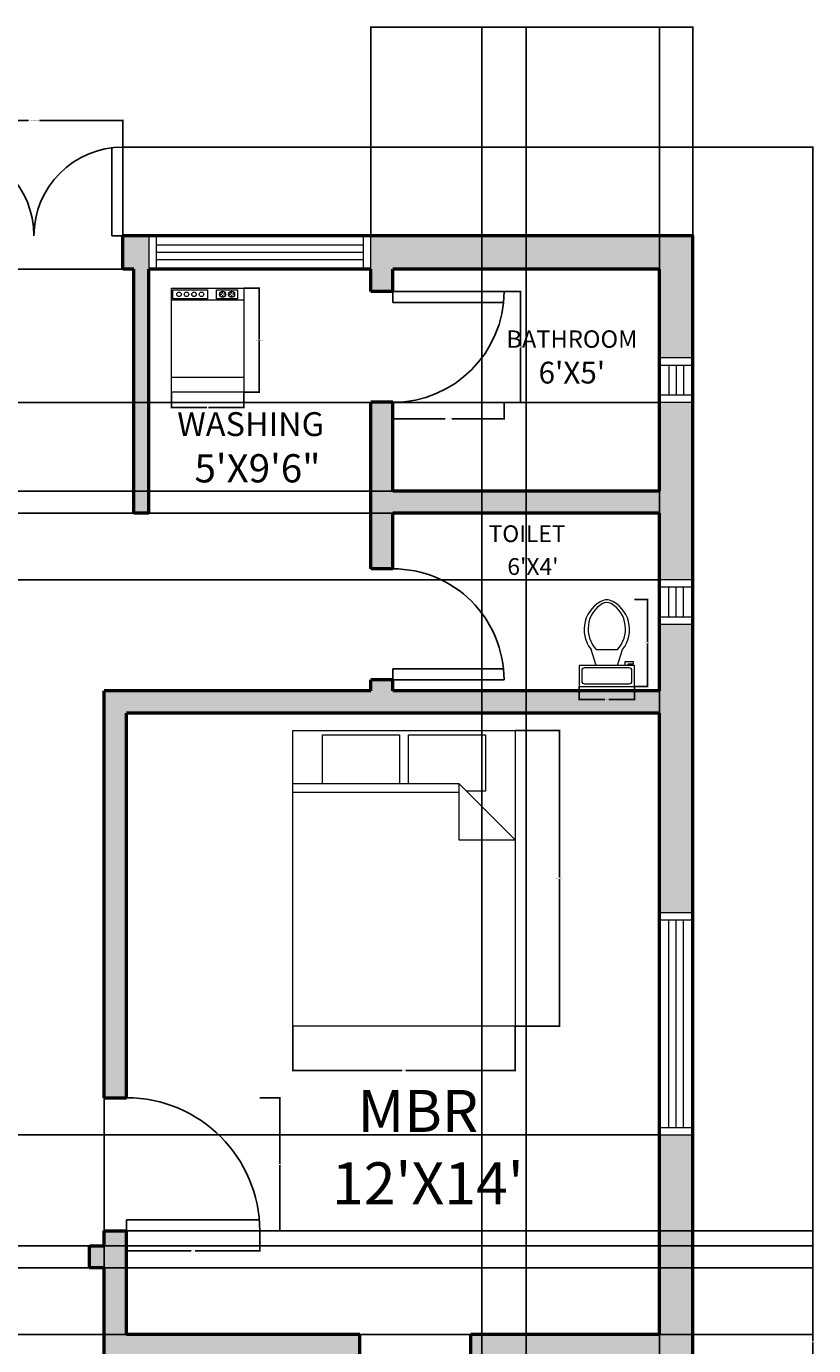
# Model space of a CAD drawing. Units: inches. Extents: x 96 to 522, y 502 to 1213.
# Tile 5 of 5: x 309 to 522, y 856 to 1213. Entities that reach past the tile are written whole.
import ezdxf

# ---------------------------------------------------------------- set-up
doc = ezdxf.new("R2010")
doc.units = ezdxf.units.IN
doc.layers.get('Defpoints').update_dxf_attribs({"color": 90})
for name, color, linetype, lineweight in [('A-ANNO-DIMS', 2, 'Continuous', 18), ('A-AREA-IDEN', 7, 'Continuous', 25), ('A-DOOR', 3, 'Continuous', 25), ('A-EQPM', 8, 'Continuous', 18), ('A-FLOR-FIXT', 9, 'Continuous', 18), ('A-FURN', 8, 'Continuous', 18), ('A-GLAZ', 4, 'Continuous', 18), ('A-WALL', 7, 'Continuous', 50)]:
    doc.layers.add(name, color=color, linetype=linetype, lineweight=lineweight)
doc.layers.add('A-WALL-PATT', color=252, linetype='Continuous', lineweight=13, true_color=0x939598)
doc.styles.get("Standard").update_dxf_attribs({"font": 'arial.ttf'})
doc.dimstyles.get("Standard").update_dxf_attribs({"dimtxt": 0.18, "dimasz": 0.18, "dimexe": 0.18, "dimexo": 0.0625, "dimgap": 0.09, "dimtad": 0, "dimtih": 1, "dimtoh": 1, "dimdec": 4, "dimzin": 0, "dimdsep": 46, "dimtxsty": 'Standard', "dimcen": 0.09, "dimadec": 0, "dimazin": 0, "dimtfac": 1, "dimtdec": 4, "dimtofl": 0, "dimtmove": 0, "dimatfit": 3, "dimfxl": 1, "dimtolj": 1, "dimtzin": 0, "dimarcsym": 0})

# ---------------------------------------------------------------- blocks, each defined once
blk = doc.blocks.new('Bed - Queen')
for p, q in [((0, -80.00003), (0, 0)), ((0, 0), (59.99999, 0)), ((59.99999, 0), (59.99999, -80.00003)), ((7.99999, -1.2), (28.79998, -1.2)), ((7.99999, -14.4), (7.99999, -1.2)), ((28.79998, -1.2), (28.79998, -14.4)), ((31.19999, -1.2), (51.99999, -1.2)), ((31.19999, -14.4), (31.19999, -1.2)), ((51.99999, -1.2), (51.99999, -16.4)), ((0, -14.4), (44.8, -14.4)), ((44.8, -16.8), (0, -16.8)), ((59.99999, -29.6), (44.8, -14.4)), ((44.8, -14.4), (44.8, -29.6)), ((51.99999, -16.4), (46.79936, -16.4)), ((44.8, -29.6), (59.99999, -29.6)), ((59.99999, -80.00003), (0, -80.00003))]:
    blk.add_line(p, q)
blk = doc.blocks.new('Toilet - top')
for p, q in [((9.5, -6), (9.5, -2)), ((-10, -8.5), (-8, -8.5)), ((-10, -9.5), (-10, -8.5)), ((-7, -9.5), (-10, -9.5)), ((-8, -8.5), (-8, -8)), ((-7, -8), (-7, -9.5)), ((-4, -8), (-6, -14)), ((4, -8), (6, -14)), ((4, -14), (-4, -14))]:
    blk.add_line(p, q)
blk.add_lwpolyline([(10.5, -8), (10.5, 0), (-10.5, 0), (-10.5, -8)], close=True)
for points in [[(-9.5, -2), (-9.5, -6)], [(8.5, -1), (-8.5, -1)], [(-8.5, -7), (8.5, -7)]]:
    blk.add_lwpolyline(points)
for centre, radius, start, end in [((-8.62, -1.88), 0.884, 81.8699, 188.1301), ((8.62, -1.88), 0.884, 351.8699, 98.1301), ((-8.62, -6.12), 0.884, 171.8699, 278.1301), ((8.62, -6.12), 0.884, 261.8699, 8.1301), ((3.52, -21.58), 12.17, 141.4691, 247.9714), ((4.2, -21.82), 11.33, 136.3677, 238.9468), ((-3.52, -21.58), 12.17, 292.0284, 38.5307), ((-4.2, -21.82), 11.33, 301.053, 43.6321), ((0, -27.88), 4, 245.7318, 294.2682), ((0, -29), 4, 254.8605, 285.1395)]:
    blk.add_arc(centre, radius, start, end)
blk = doc.blocks.new('Dishwasher')
for p, q in [((16, 32.5), (16.75, 32.5)), ((16.5, 32), (16.2942, 31.7942)), ((16.3156, 33.1843), (16.5, 33)), ((17, 32.75), (17, 33.5)), ((17, 32.25), (17, 31.5)), ((18, 32.5), (17.25, 32.5)), ((17.5, 33), (17.6938, 33.1938)), ((17.7061, 31.7939), (17.5, 32)), ((19, 32.5), (19.75, 32.5)), ((19.5, 32), (19.2942, 31.7942)), ((19.3156, 33.1843), (19.5, 33)), ((20, 32.75), (20, 33.5)), ((20, 32.25), (20, 31.5)), ((21, 32.5), (20.25, 32.5)), ((20.5, 33), (20.6938, 33.1938)), ((20.7061, 31.7939), (20.5, 32)), ((24, 30.5), (0, 30.5)), ((0, 5), (24, 5))]:
    blk.add_line(p, q)
for points in [[(0, 0), (0, 34.5), (24, 34.5), (24, 0)], [(0.5, 31), (0.5, 34), (12, 34), (12, 31)], [(15, 31), (15, 34), (22, 34), (22, 31)]]:
    blk.add_lwpolyline(points, close=True)
for centre, radius in [((2.5, 32.5), 0.75), ((5, 32.5), 0.75), ((7.5, 32.5), 0.75), ((10, 32.5), 0.75), ((17, 32.5), 1), ((20, 32.5), 1)]:
    blk.add_circle(centre, radius)
blk = doc.blocks.new('WIN-60IN')
for p, q in [((60, 9), (0, 9)), ((0, 9), (0, 0)), ((2, 9), (2, 0)), ((58, 0), (58, 9)), ((60, 0), (60, 9)), ((2, 6.5), (58, 6.5)), ((2, 4.5), (58, 4.5)), ((0, 0), (60, 0)), ((2, 2.5), (58, 2.5))]:
    blk.add_line(p, q)
blk = doc.blocks.new('WIN-12IN')
for p, q in [((0, 12), (0, 0)), ((9, 12), (0, 12)), ((9, 0), (9, 12)), ((9, 10), (0, 10)), ((2.5, 10), (2.5, 2)), ((4.5, 10), (4.5, 2)), ((6.5, 10), (6.5, 2)), ((0, 2), (9, 2)), ((0, 0), (9, 0))]:
    blk.add_line(p, q)
blk = doc.blocks.new('DOOR-SGL-36IN')
for p, q in [((36, 3), (0, 3)), ((0, 0), (0, 3)), ((36, 0), (0, 0))]:
    blk.add_line(p, q)
blk.add_arc((0, 0), 36, 0, 90)
blk = doc.blocks.new('DOOR-SGL-30IN')
for p, q in [((30, 30), (0, 30)), ((0, 30), (0, 27)), ((30, 27), (0, 27))]:
    blk.add_line(p, q)
blk.add_arc((0, 30), 30, 270, 0)
blk = doc.blocks.new('DOOR-DBL-48IN')
for p, q in [((0, 24), (0, 0)), ((3, 24), (3, 0)), ((45, 24), (45, 0)), ((48, 24), (48, 0)), ((0, 0), (3, 0)), ((48, 0), (45, 0))]:
    blk.add_line(p, q)
for centre, start, end in [((0, 0), 0, 90), ((48, 0), 90, 180)]:
    blk.add_arc(centre, 24, start, end)
blk = doc.blocks.new('*D21')
at = {"layer": 'A-ANNO-DIMS', "color": 0, "lineweight": -2, "transparency": 16777216}
for p, q in [((408.21, 1111.19), (408.21, 1106.57)), ((438.21, 1111.19), (438.21, 1106.57)), ((408.39, 1106.75), (422.28, 1106.75)), ((438.03, 1106.75), (424.15, 1106.75))]:
    blk.add_line(p, q, dxfattribs=at)
at = {"layer": 'A-ANNO-DIMS', "color": 0, "transparency": 16777216}
for points in [[(408.39, 1106.78), (408.39, 1106.72), (408.21, 1106.75)], [(438.03, 1106.78), (438.03, 1106.72), (438.21, 1106.75)]]:
    blk.add_solid(points, dxfattribs=at)
at = {"layer": 'Defpoints', "color": 0, "transparency": 16777216}
for p in [(408.21, 1111.25), (438.21, 1111.25), (438.21, 1106.75)]:
    blk.add_point(p, dxfattribs=at)
at = {"layer": 'A-ANNO-DIMS', "color": 0, "transparency": 16777216, "insert": (423.21, 1106.75), "char_height": 0.18, "attachment_point": 5}
blk.add_mtext('\\A1;DOOR 30 TYP.', dxfattribs=at)
blk = doc.blocks.new('*D22')
at = {"layer": 'A-ANNO-DIMS', "color": 0, "lineweight": -2, "transparency": 16777216}
for p, q in [((438.27, 1141.25), (442.89, 1141.25)), ((442.71, 1141.07), (442.71, 1126.43)), ((442.71, 1111.43), (442.71, 1126.07)), ((438.27, 1111.25), (442.89, 1111.25))]:
    blk.add_line(p, q, dxfattribs=at)
at = {"layer": 'A-ANNO-DIMS', "color": 0, "transparency": 16777216}
for points in [[(442.68, 1141.07), (442.74, 1141.07), (442.71, 1141.25)], [(442.68, 1111.43), (442.74, 1111.43), (442.71, 1111.25)]]:
    blk.add_solid(points, dxfattribs=at)
at = {"layer": 'Defpoints', "color": 0, "transparency": 16777216}
for p in [(438.21, 1141.25), (442.71, 1141.25), (438.21, 1111.25)]:
    blk.add_point(p, dxfattribs=at)
at = {"layer": 'A-ANNO-DIMS', "color": 0, "transparency": 16777216, "insert": (442.71, 1126.25), "char_height": 0.18, "attachment_point": 5}
blk.add_mtext('\\A1;30 TYP.', dxfattribs=at)
blk = doc.blocks.new('*D23')
at = {"layer": 'A-ANNO-DIMS', "color": 0, "lineweight": -2, "transparency": 16777216}
for p, q in [((372.27, 923.25), (377.79, 923.25)), ((377.61, 923.07), (377.61, 905.43)), ((377.61, 887.43), (377.61, 905.07)), ((372.27, 887.25), (377.79, 887.25))]:
    blk.add_line(p, q, dxfattribs=at)
at = {"layer": 'A-ANNO-DIMS', "color": 0, "transparency": 16777216}
for points in [[(377.58, 923.07), (377.64, 923.07), (377.61, 923.25)], [(377.58, 887.43), (377.64, 887.43), (377.61, 887.25)]]:
    blk.add_solid(points, dxfattribs=at)
at = {"layer": 'Defpoints', "color": 0, "transparency": 16777216}
for p in [(372.21, 923.25), (377.61, 923.25), (372.21, 887.25)]:
    blk.add_point(p, dxfattribs=at)
at = {"layer": 'A-ANNO-DIMS', "color": 0, "transparency": 16777216, "insert": (377.61, 905.25), "char_height": 0.18, "attachment_point": 5}
blk.add_mtext('\\A1;DOOR 36 TYP.', dxfattribs=at)
blk = doc.blocks.new('*D24')
at = {"layer": 'A-ANNO-DIMS', "color": 0, "lineweight": -2, "transparency": 16777216}
for p, q in [((336.21, 887.19), (336.21, 881.67)), ((372.21, 887.19), (372.21, 881.67)), ((336.39, 881.85), (353.68, 881.85)), ((372.03, 881.85), (354.74, 881.85))]:
    blk.add_line(p, q, dxfattribs=at)
at = {"layer": 'A-ANNO-DIMS', "color": 0, "transparency": 16777216}
for points in [[(336.39, 881.88), (336.39, 881.82), (336.21, 881.85)], [(372.03, 881.88), (372.03, 881.82), (372.21, 881.85)]]:
    blk.add_solid(points, dxfattribs=at)
at = {"layer": 'Defpoints', "color": 0, "transparency": 16777216}
for p in [(336.21, 887.25), (372.21, 887.25), (372.21, 881.85)]:
    blk.add_point(p, dxfattribs=at)
at = {"layer": 'A-ANNO-DIMS', "color": 0, "transparency": 16777216, "insert": (354.21, 881.85), "char_height": 0.18, "attachment_point": 5}
blk.add_mtext('\\A1;36 TYP.', dxfattribs=at)
blk = doc.blocks.new('*D25')
at = {"layer": 'A-ANNO-DIMS', "color": 0, "lineweight": -2, "transparency": 16777216}
for p, q in [((287.21, 1180.31), (287.21, 1187.63)), ((335.21, 1180.31), (335.21, 1187.63)), ((287.39, 1187.45), (309.72, 1187.45)), ((335.03, 1187.45), (312.7, 1187.45))]:
    blk.add_line(p, q, dxfattribs=at)
at = {"layer": 'A-ANNO-DIMS', "color": 0, "transparency": 16777216}
for points in [[(287.39, 1187.48), (287.39, 1187.42), (287.21, 1187.45)], [(335.03, 1187.48), (335.03, 1187.42), (335.21, 1187.45)]]:
    blk.add_solid(points, dxfattribs=at)
at = {"layer": 'Defpoints', "color": 0, "transparency": 16777216}
for p in [(335.21, 1187.45), (287.21, 1180.25), (335.21, 1180.25)]:
    blk.add_point(p, dxfattribs=at)
at = {"layer": 'A-ANNO-DIMS', "color": 0, "transparency": 16777216, "insert": (311.21, 1187.45), "char_height": 0.18, "attachment_point": 5}
blk.add_mtext('\\A1;DOUBLE DOOR 48 TYP.', dxfattribs=at)
blk = doc.blocks.new('*D27')
at = {"layer": 'A-ANNO-DIMS', "color": 0, "lineweight": -2, "transparency": 16777216}
for p, q in [((441.25, 1022.58), (453.37, 1022.58)), ((453.19, 1022.4), (453.19, 982.77)), ((453.19, 942.76), (453.19, 982.39)), ((441.25, 942.58), (453.37, 942.58))]:
    blk.add_line(p, q, dxfattribs=at)
at = {"layer": 'A-ANNO-DIMS', "color": 0, "transparency": 16777216}
for points in [[(453.16, 1022.4), (453.22, 1022.4), (453.19, 1022.58)], [(453.16, 942.76), (453.22, 942.76), (453.19, 942.58)]]:
    blk.add_solid(points, dxfattribs=at)
at = {"layer": 'Defpoints', "color": 0, "transparency": 16777216}
for p in [(441.19, 1022.58), (453.19, 1022.58), (441.19, 942.58)]:
    blk.add_point(p, dxfattribs=at)
at = {"layer": 'A-ANNO-DIMS', "color": 0, "transparency": 16777216, "insert": (453.19, 982.58), "char_height": 0.18, "attachment_point": 5}
blk.add_mtext('\\A1;QUEEN BED 80 TYP.', dxfattribs=at)
blk = doc.blocks.new('*D28')
at = {"layer": 'A-ANNO-DIMS', "color": 0, "lineweight": -2, "transparency": 16777216}
for p, q in [((381.19, 942.52), (381.19, 930.4)), ((441.19, 942.52), (441.19, 930.4)), ((381.37, 930.58), (410.66, 930.58)), ((441.01, 930.58), (411.72, 930.58))]:
    blk.add_line(p, q, dxfattribs=at)
at = {"layer": 'A-ANNO-DIMS', "color": 0, "transparency": 16777216}
for points in [[(381.37, 930.61), (381.37, 930.55), (381.19, 930.58)], [(441.01, 930.61), (441.01, 930.55), (441.19, 930.58)]]:
    blk.add_solid(points, dxfattribs=at)
at = {"layer": 'Defpoints', "color": 0, "transparency": 16777216}
for p in [(381.19, 942.58), (441.19, 942.58), (441.19, 930.58)]:
    blk.add_point(p, dxfattribs=at)
at = {"layer": 'A-ANNO-DIMS', "color": 0, "transparency": 16777216, "insert": (411.19, 930.58), "char_height": 0.18, "attachment_point": 5}
blk.add_mtext('\\A1;60 TYP.', dxfattribs=at)
blk = doc.blocks.new('*D29')
at = {"layer": 'A-ANNO-DIMS', "color": 0, "lineweight": -2, "transparency": 16777216}
for p, q in [((473.51, 1057.93), (477.15, 1057.93)), ((476.97, 1057.75), (476.97, 1046.39)), ((476.97, 1034.65), (476.97, 1046.02)), ((473.51, 1034.47), (477.15, 1034.47))]:
    blk.add_line(p, q, dxfattribs=at)
at = {"layer": 'A-ANNO-DIMS', "color": 0, "transparency": 16777216}
for points in [[(476.94, 1057.75), (477, 1057.75), (476.97, 1057.93)], [(476.94, 1034.65), (477, 1034.65), (476.97, 1034.47)]]:
    blk.add_solid(points, dxfattribs=at)
at = {"layer": 'Defpoints', "color": 0, "transparency": 16777216}
for p in [(473.45, 1057.93), (473.45, 1034.47), (476.97, 1034.47)]:
    blk.add_point(p, dxfattribs=at)
at = {"layer": 'A-ANNO-DIMS', "color": 0, "transparency": 16777216, "insert": (476.97, 1046.2), "char_height": 0.18, "attachment_point": 5}
blk.add_mtext('\\A1;WC 23 TYP.', dxfattribs=at)
blk = doc.blocks.new('*D30')
at = {"layer": 'A-ANNO-DIMS', "color": 0, "lineweight": -2, "transparency": 16777216}
for p, q in [((458.54, 1034.41), (458.54, 1030.77)), ((473.45, 1034.41), (473.45, 1030.77)), ((458.72, 1030.95), (465.48, 1030.95)), ((473.27, 1030.95), (466.51, 1030.95))]:
    blk.add_line(p, q, dxfattribs=at)
at = {"layer": 'A-ANNO-DIMS', "color": 0, "transparency": 16777216}
for points in [[(458.72, 1030.98), (458.72, 1030.92), (458.54, 1030.95)], [(473.27, 1030.98), (473.27, 1030.92), (473.45, 1030.95)]]:
    blk.add_solid(points, dxfattribs=at)
at = {"layer": 'Defpoints', "color": 0, "transparency": 16777216}
for p in [(458.54, 1034.47), (473.45, 1034.47), (458.54, 1030.95)]:
    blk.add_point(p, dxfattribs=at)
at = {"layer": 'A-ANNO-DIMS', "color": 0, "transparency": 16777216, "insert": (466, 1030.95), "char_height": 0.18, "attachment_point": 5}
blk.add_mtext('\\A1;15 TYP.', dxfattribs=at)
blk = doc.blocks.new('*D43')
at = {"layer": 'A-ANNO-DIMS', "color": 0, "lineweight": -2, "transparency": 16777216}
for p, q in [((367.93, 1142.08), (372.26, 1142.08)), ((372.08, 1141.9), (372.08, 1128.23)), ((372.08, 1114.2), (372.08, 1127.87)), ((367.93, 1114.02), (372.26, 1114.02))]:
    blk.add_line(p, q, dxfattribs=at)
at = {"layer": 'A-ANNO-DIMS', "color": 0, "transparency": 16777216}
for points in [[(372.05, 1141.9), (372.11, 1141.9), (372.08, 1142.08)], [(372.05, 1114.2), (372.11, 1114.2), (372.08, 1114.02)]]:
    blk.add_solid(points, dxfattribs=at)
at = {"layer": 'Defpoints', "color": 0, "transparency": 16777216}
for p in [(367.87, 1142.08), (372.08, 1142.08), (367.87, 1114.02)]:
    blk.add_point(p, dxfattribs=at)
at = {"layer": 'A-ANNO-DIMS', "color": 0, "transparency": 16777216, "insert": (372.08, 1128.05), "char_height": 0.18, "attachment_point": 5}
blk.add_mtext('\\A1;DISHWASHER 28', dxfattribs=at)
blk = doc.blocks.new('*D44')
at = {"layer": 'A-ANNO-DIMS', "color": 0, "lineweight": -2, "transparency": 16777216}
for p, q in [((348.35, 1113.96), (348.35, 1109.63)), ((367.87, 1113.96), (367.87, 1109.63)), ((348.53, 1109.81), (357.89, 1109.81)), ((367.69, 1109.81), (358.33, 1109.81))]:
    blk.add_line(p, q, dxfattribs=at)
at = {"layer": 'A-ANNO-DIMS', "color": 0, "transparency": 16777216}
for points in [[(348.53, 1109.84), (348.53, 1109.78), (348.35, 1109.81)], [(367.69, 1109.84), (367.69, 1109.78), (367.87, 1109.81)]]:
    blk.add_solid(points, dxfattribs=at)
at = {"layer": 'Defpoints', "color": 0, "transparency": 16777216}
for p in [(348.35, 1114.02), (367.87, 1114.02), (367.87, 1109.81)]:
    blk.add_point(p, dxfattribs=at)
at = {"layer": 'A-ANNO-DIMS', "color": 0, "transparency": 16777216, "insert": (358.11, 1109.81), "char_height": 0.18, "attachment_point": 5}
blk.add_mtext('\\A1;20', dxfattribs=at)
blk = doc.blocks.new('*D48')
at = {"layer": 'A-ANNO-DIMS', "color": 0, "lineweight": -2, "transparency": 16777216}
for p, q in [((335.27, 1180.25), (521.84, 1180.25)), ((521.66, 1180.07), (521.66, 857.43)), ((521.66, 534.43), (521.66, 857.07)), ((489.27, 534.25), (521.84, 534.25))]:
    blk.add_line(p, q, dxfattribs=at)
at = {"layer": 'A-ANNO-DIMS', "color": 0, "transparency": 16777216}
for points in [[(521.63, 1180.07), (521.69, 1180.07), (521.66, 1180.25)], [(521.63, 534.43), (521.69, 534.43), (521.66, 534.25)]]:
    blk.add_solid(points, dxfattribs=at)
at = {"layer": 'Defpoints', "color": 0, "transparency": 16777216}
for p in [(335.21, 1180.25), (521.66, 1180.25), (489.21, 534.25)]:
    blk.add_point(p, dxfattribs=at)
at = {"layer": 'A-ANNO-DIMS', "color": 0, "transparency": 16777216, "insert": (521.66, 857.25), "char_height": 0.18, "attachment_point": 5}
blk.add_mtext('\\A1;646', dxfattribs=at)
blk = doc.blocks.new('*D52')
at = {"layer": 'A-ANNO-DIMS', "color": 0, "lineweight": -2, "transparency": 16777216}
for p, q in [((402.21, 1156.31), (402.21, 1212.88)), ((402.39, 1212.7), (445.49, 1212.7)), ((489.03, 1212.7), (445.93, 1212.7)), ((489.21, 1156.31), (489.21, 1212.88))]:
    blk.add_line(p, q, dxfattribs=at)
at = {"layer": 'A-ANNO-DIMS', "color": 0, "transparency": 16777216}
for points in [[(402.39, 1212.73), (402.39, 1212.67), (402.21, 1212.7)], [(489.03, 1212.73), (489.03, 1212.67), (489.21, 1212.7)]]:
    blk.add_solid(points, dxfattribs=at)
at = {"layer": 'Defpoints', "color": 0, "transparency": 16777216}
for p in [(489.21, 1212.7), (402.21, 1156.25), (489.21, 1156.25)]:
    blk.add_point(p, dxfattribs=at)
at = {"layer": 'A-ANNO-DIMS', "color": 0, "transparency": 16777216, "insert": (445.71, 1212.7), "char_height": 0.18, "attachment_point": 5}
blk.add_mtext('\\A1;87', dxfattribs=at)
blk = doc.blocks.new('*D55')
at = {"layer": 'A-ANNO-DIMS', "color": 0, "lineweight": -2, "transparency": 16777216}
for p, q in [((432.21, 661.31), (432.21, 1212.88)), ((432.39, 1212.7), (455.99, 1212.7)), ((480.03, 1212.7), (456.43, 1212.7)), ((480.21, 661.31), (480.21, 1212.88))]:
    blk.add_line(p, q, dxfattribs=at)
at = {"layer": 'A-ANNO-DIMS', "color": 0, "transparency": 16777216}
for points in [[(432.39, 1212.73), (432.39, 1212.67), (432.21, 1212.7)], [(480.03, 1212.73), (480.03, 1212.67), (480.21, 1212.7)]]:
    blk.add_solid(points, dxfattribs=at)
at = {"layer": 'Defpoints', "color": 0, "transparency": 16777216}
for p in [(480.21, 1212.7), (432.21, 661.25), (480.21, 661.25)]:
    blk.add_point(p, dxfattribs=at)
at = {"layer": 'A-ANNO-DIMS', "color": 0, "transparency": 16777216, "insert": (456.21, 1212.7), "char_height": 0.18, "attachment_point": 5}
blk.add_mtext('\\A1;48', dxfattribs=at)
blk = doc.blocks.new('*D62')
at = {"layer": 'A-ANNO-DIMS', "color": 0, "lineweight": -2, "transparency": 16777216}
for p, q in [((480.15, 913.25), (96.58, 913.25)), ((96.76, 913.07), (96.76, 886.43)), ((96.76, 859.43), (96.76, 886.07)), ((480.15, 859.25), (96.58, 859.25))]:
    blk.add_line(p, q, dxfattribs=at)
at = {"layer": 'A-ANNO-DIMS', "color": 0, "transparency": 16777216}
for points in [[(96.73, 913.07), (96.79, 913.07), (96.76, 913.25)], [(96.73, 859.43), (96.79, 859.43), (96.76, 859.25)]]:
    blk.add_solid(points, dxfattribs=at)
at = {"layer": 'Defpoints', "color": 0, "transparency": 16777216}
for p in [(96.76, 913.25), (480.21, 913.25), (480.21, 859.25)]:
    blk.add_point(p, dxfattribs=at)
at = {"layer": 'A-ANNO-DIMS', "color": 0, "transparency": 16777216, "insert": (96.76, 886.25), "char_height": 0.18, "attachment_point": 5}
blk.add_mtext('\\A1;54', dxfattribs=at)
blk = doc.blocks.new('*D63')
at = {"layer": 'A-ANNO-DIMS', "color": 0, "lineweight": -2, "transparency": 16777216}
for p, q in [((480.15, 1081.25), (96.58, 1081.25)), ((96.76, 1081.07), (96.76, 1072.43)), ((96.76, 1063.43), (96.76, 1072.07)), ((480.15, 1063.25), (96.58, 1063.25))]:
    blk.add_line(p, q, dxfattribs=at)
at = {"layer": 'A-ANNO-DIMS', "color": 0, "transparency": 16777216}
for points in [[(96.73, 1081.07), (96.79, 1081.07), (96.76, 1081.25)], [(96.73, 1063.43), (96.79, 1063.43), (96.76, 1063.25)]]:
    blk.add_solid(points, dxfattribs=at)
at = {"layer": 'Defpoints', "color": 0, "transparency": 16777216}
for p in [(96.76, 1081.25), (480.21, 1081.25), (480.21, 1063.25)]:
    blk.add_point(p, dxfattribs=at)
at = {"layer": 'A-ANNO-DIMS', "color": 0, "transparency": 16777216, "insert": (96.76, 1072.25), "char_height": 0.18, "attachment_point": 5}
blk.add_mtext('\\A1;18', dxfattribs=at)
blk = doc.blocks.new('*D64')
at = {"layer": 'A-ANNO-DIMS', "color": 0, "lineweight": -2, "transparency": 16777216}
for p, q in [((480.15, 1111.25), (96.58, 1111.25)), ((96.76, 1111.07), (96.76, 1099.43)), ((96.76, 1087.43), (96.76, 1099.07)), ((480.15, 1087.25), (96.58, 1087.25))]:
    blk.add_line(p, q, dxfattribs=at)
at = {"layer": 'A-ANNO-DIMS', "color": 0, "transparency": 16777216}
for points in [[(96.73, 1111.07), (96.79, 1111.07), (96.76, 1111.25)], [(96.73, 1087.43), (96.79, 1087.43), (96.76, 1087.25)]]:
    blk.add_solid(points, dxfattribs=at)
at = {"layer": 'Defpoints', "color": 0, "transparency": 16777216}
for p in [(96.76, 1111.25), (480.21, 1111.25), (480.21, 1087.25)]:
    blk.add_point(p, dxfattribs=at)
at = {"layer": 'A-ANNO-DIMS', "color": 0, "transparency": 16777216, "insert": (96.76, 1099.25), "char_height": 0.18, "attachment_point": 5}
blk.add_mtext('\\A1;24', dxfattribs=at)
blk = doc.blocks.new('*D65')
at = {"layer": 'A-ANNO-DIMS', "color": 0, "lineweight": -2, "transparency": 16777216}
for p, q in [((444.21, 543.31), (444.21, 1212.88)), ((444.39, 1212.7), (461.99, 1212.7)), ((480.03, 1212.7), (462.43, 1212.7)), ((480.21, 543.31), (480.21, 1212.88))]:
    blk.add_line(p, q, dxfattribs=at)
at = {"layer": 'A-ANNO-DIMS', "color": 0, "transparency": 16777216}
for points in [[(444.39, 1212.73), (444.39, 1212.67), (444.21, 1212.7)], [(480.03, 1212.73), (480.03, 1212.67), (480.21, 1212.7)]]:
    blk.add_solid(points, dxfattribs=at)
at = {"layer": 'Defpoints', "color": 0, "transparency": 16777216}
for p in [(480.21, 1212.7), (444.21, 543.25), (480.21, 543.25)]:
    blk.add_point(p, dxfattribs=at)
at = {"layer": 'A-ANNO-DIMS', "color": 0, "transparency": 16777216, "insert": (462.21, 1212.7), "char_height": 0.18, "attachment_point": 5}
blk.add_mtext('\\A1;36', dxfattribs=at)
blk = doc.blocks.new('*D66')
at = {"layer": 'A-ANNO-DIMS', "color": 0, "lineweight": -2, "transparency": 16777216}
for p, q in [((330.21, 1033.19), (330.21, 501.62)), ((276.21, 997.19), (276.21, 501.62)), ((276.39, 501.8), (302.99, 501.8)), ((330.03, 501.8), (303.43, 501.8))]:
    blk.add_line(p, q, dxfattribs=at)
at = {"layer": 'A-ANNO-DIMS', "color": 0, "transparency": 16777216}
for points in [[(276.39, 501.83), (276.39, 501.77), (276.21, 501.8)], [(330.03, 501.83), (330.03, 501.77), (330.21, 501.8)]]:
    blk.add_solid(points, dxfattribs=at)
at = {"layer": 'Defpoints', "color": 0, "transparency": 16777216}
for p in [(330.21, 1033.25), (276.21, 997.25), (330.21, 501.8)]:
    blk.add_point(p, dxfattribs=at)
at = {"layer": 'A-ANNO-DIMS', "color": 0, "transparency": 16777216, "insert": (303.21, 501.8), "char_height": 0.18, "attachment_point": 5}
blk.add_mtext('\\A1;54', dxfattribs=at)
blk = doc.blocks.new('*D67')
at = {"layer": 'A-ANNO-DIMS', "color": 0, "lineweight": -2, "transparency": 16777216}
for p, q in [((276.27, 883.25), (521.84, 883.25)), ((521.66, 883.07), (521.66, 880.43)), ((521.66, 877.43), (521.66, 880.07)), ((276.27, 877.25), (521.84, 877.25))]:
    blk.add_line(p, q, dxfattribs=at)
at = {"layer": 'A-ANNO-DIMS', "color": 0, "transparency": 16777216}
for points in [[(521.63, 883.07), (521.69, 883.07), (521.66, 883.25)], [(521.63, 877.43), (521.69, 877.43), (521.66, 877.25)]]:
    blk.add_solid(points, dxfattribs=at)
at = {"layer": 'Defpoints', "color": 0, "transparency": 16777216}
for p in [(276.21, 883.25), (521.66, 883.25), (276.21, 877.25)]:
    blk.add_point(p, dxfattribs=at)
at = {"layer": 'A-ANNO-DIMS', "color": 0, "transparency": 16777216, "insert": (521.66, 880.25), "char_height": 0.18, "attachment_point": 5}
blk.add_mtext('\\A1;6', dxfattribs=at)
blk = doc.blocks.new('*D68')
at = {"layer": 'A-ANNO-DIMS', "color": 0, "lineweight": -2, "transparency": 16777216}
for p, q in [((336.27, 887.25), (521.84, 887.25)), ((521.66, 887.07), (521.66, 873.43)), ((521.66, 859.43), (521.66, 873.07)), ((336.27, 859.25), (521.84, 859.25))]:
    blk.add_line(p, q, dxfattribs=at)
at = {"layer": 'A-ANNO-DIMS', "color": 0, "transparency": 16777216}
for points in [[(521.63, 887.07), (521.69, 887.07), (521.66, 887.25)], [(521.63, 859.43), (521.69, 859.43), (521.66, 859.25)]]:
    blk.add_solid(points, dxfattribs=at)
at = {"layer": 'Defpoints', "color": 0, "transparency": 16777216}
for p in [(336.21, 887.25), (521.66, 887.25), (336.21, 859.25)]:
    blk.add_point(p, dxfattribs=at)
at = {"layer": 'A-ANNO-DIMS', "color": 0, "transparency": 16777216, "insert": (521.66, 873.25), "char_height": 0.18, "attachment_point": 5}
blk.add_mtext('\\A1;28', dxfattribs=at)
blk = doc.blocks.new('*D71')
at = {"layer": 'A-ANNO-DIMS', "color": 0, "lineweight": -2, "transparency": 16777216}
for p, q in [((338.15, 1147.25), (96.58, 1147.25)), ((96.76, 1147.07), (96.76, 1114.43)), ((96.76, 1081.43), (96.76, 1114.07)), ((338.15, 1081.25), (96.58, 1081.25))]:
    blk.add_line(p, q, dxfattribs=at)
at = {"layer": 'A-ANNO-DIMS', "color": 0, "transparency": 16777216}
for points in [[(96.73, 1147.07), (96.79, 1147.07), (96.76, 1147.25)], [(96.73, 1081.43), (96.79, 1081.43), (96.76, 1081.25)]]:
    blk.add_solid(points, dxfattribs=at)
at = {"layer": 'Defpoints', "color": 0, "transparency": 16777216}
for p in [(96.76, 1147.25), (338.21, 1147.25), (338.21, 1081.25)]:
    blk.add_point(p, dxfattribs=at)
at = {"layer": 'A-ANNO-DIMS', "color": 0, "transparency": 16777216, "insert": (96.76, 1114.25), "char_height": 0.18, "attachment_point": 5}
blk.add_mtext('\\A1;66', dxfattribs=at)

msp = doc.modelspace()

# ---------------------------------------------------------------- hatches: boundary and pattern name
at = {"layer": 'A-WALL-PATT'}
h = msp.add_hatch(color=256, dxfattribs=at)
h.dxf.hatch_style = 1
h.paths.add_polyline_path([(174.2111, 1156.2511), (129.2111, 1156.2511), (129.2111, 1105.2511), (138.2111, 1105.2511), (138.2111, 1147.2511), (174.2111, 1147.2511)])
h.paths.add_polyline_path([(287.2111, 1156.2511), (234.2111, 1156.2511), (234.2111, 1147.2511), (270.2111, 1147.2511), (270.2111, 1003.2511), (267.2111, 1003.2511), (267.2111, 997.2511), (276.2111, 997.2511), (276.2111, 1147.2511), (287.2111, 1147.2511)])
h.paths.add_polyline_path([(342.2111, 1156.2511), (335.2111, 1156.2511), (335.2111, 1147.2511), (338.2111, 1147.2511), (338.2111, 1081.2511), (342.2111, 1081.2511), (342.2111, 1147.2511)])
h.paths.add_polyline_path([(489.2111, 1156.2511), (402.2111, 1156.2511), (402.2111, 1147.2511), (402.2111, 1141.2511), (408.2111, 1141.2511), (408.2111, 1147.2511), (480.2111, 1147.2511), (480.2111, 1123.2511), (489.2111, 1123.2511)])
h.paths.add_polyline_path([(489.2111, 1111.2511), (480.2111, 1111.2511), (480.2111, 1087.2511), (408.2111, 1087.2511), (408.2111, 1111.2511), (402.2111, 1111.2511), (402.2111, 1066.2511), (408.2111, 1066.2511), (408.2111, 1081.2511), (480.2111, 1081.2511), (480.2111, 1063.2511), (489.2111, 1063.2511)])
h.paths.add_polyline_path([(489.2111, 1051.2511), (480.2111, 1051.2511), (480.2111, 1033.2511), (408.2111, 1033.2511), (408.2111, 1036.2511), (402.2111, 1036.2511), (402.2111, 1033.2511), (338.2111, 1033.2511), (330.2111, 1033.2511), (330.2111, 923.2511), (336.2111, 923.2511), (336.2111, 1027.2511), (338.2111, 1027.2511), (402.2111, 1027.2511), (480.2111, 1027.2511), (480.2111, 973.2511), (489.2111, 973.2511)])
h.paths.add_polyline_path([(489.2111, 913.2511), (480.2111, 913.2511), (480.2111, 859.2511), (429.2111, 859.2511), (429.2111, 853.2511), (480.2111, 853.2511), (480.2111, 829.2511), (489.2111, 829.2511)])
h.paths.add_polyline_path([(489.2111, 817.2511), (480.2111, 817.2511), (480.2111, 793.2511), (402.2111, 793.2511), (396.2111, 793.2511), (396.2111, 853.2511), (399.2111, 853.2511), (399.2111, 859.2511), (338.2111, 859.2511), (336.2111, 859.2511), (336.2111, 877.2511), (336.2111, 883.2511), (336.2111, 887.2511), (330.2111, 887.2511), (330.2111, 883.2511), (326.2111, 883.2511), (326.2111, 877.2511), (330.2111, 877.2511), (330.2111, 853.2511), (338.2111, 853.2511), (390.2111, 853.2511), (390.2111, 793.2511), (387.2111, 793.2511), (387.2111, 787.2511), (402.2111, 787.2511), (480.2111, 787.2511), (480.2111, 754.2511), (489.2111, 754.2511)])
h.paths.add_polyline_path([(489.2111, 694.2511), (480.2111, 694.2511), (480.2111, 661.2511), (432.2111, 661.2511), (432.2111, 652.2511), (480.2111, 652.2511), (480.2111, 543.2511), (333.2111, 543.2511), (333.2111, 534.2511), (489.2111, 534.2511), (489.2111, 652.2511)])
h.paths.add_polyline_path([(372.2111, 661.2511), (336.2111, 661.2511), (336.2111, 787.2511), (338.2111, 787.2511), (351.2111, 787.2511), (351.2111, 793.2511), (338.2111, 793.2511), (330.2111, 793.2511), (330.2111, 661.2511), (324.2111, 661.2511), (324.2111, 652.2511), (372.2111, 652.2511)])
h.paths.add_polyline_path([(138.2111, 680.6946), (129.2111, 680.6946), (129.2111, 652.2511), (177.2111, 652.2511), (177.2111, 661.2511), (138.2111, 661.2511)])
h.paths.add_polyline_path([(276.2111, 661.2511), (237.2111, 661.2511), (237.2111, 652.2511), (276.2111, 652.2511)])
h.paths.add_polyline_path([(138.2111, 803.1393), (129.2111, 803.1393), (129.2111, 740.6946), (138.2111, 740.6946)])
h.paths.add_polyline_path([(138.2111, 907.2511), (129.2111, 907.2511), (129.2111, 863.1393), (138.2111, 863.1393), (138.2111, 877.2511), (276.2111, 877.2511), (276.2111, 883.2511), (204.2111, 883.2511), (204.2111, 886.2511), (198.2111, 886.2511), (198.2111, 883.2511), (138.2111, 883.2511)])
h.paths.add_polyline_path([(138.2111, 943.2511), (198.2111, 943.2511), (198.2111, 916.2511), (204.2111, 916.2511), (204.2111, 949.2511), (138.2111, 949.2511), (138.2111, 997.2511), (231.2111, 997.2511), (231.2111, 1003.2511), (138.2111, 1003.2511), (138.2111, 1045.2511), (129.2111, 1045.2511), (129.2111, 919.2511), (138.2111, 919.2511)])

# ---------------------------------------------------------------- linework, layer by layer
at = {"layer": 'A-WALL'}
for p, q in [((335.2111, 1147.2511), (335.2111, 1156.2511)), ((338.2111, 1147.2511), (335.2111, 1147.2511)), ((338.2111, 1081.2511), (338.2111, 1147.2511)), ((342.2111, 1081.2511), (342.2111, 1147.2511)), ((402.2111, 1147.2511), (342.2111, 1147.2511)), ((402.2111, 1141.2511), (402.2111, 1147.2511)), ((480.2111, 1147.2511), (408.2111, 1147.2511)), ((408.2111, 1141.2511), (408.2111, 1147.2511)), ((480.2111, 1087.2511), (480.2111, 1147.2511)), ((408.2111, 1141.2511), (402.2111, 1141.2511)), ((408.2111, 1111.2511), (402.2111, 1111.2511)), ((402.2111, 1066.2511), (402.2111, 1111.2511)), ((408.2111, 1087.2511), (408.2111, 1111.2511)), ((480.2111, 1087.2511), (408.2111, 1087.2511)), ((342.2111, 1081.2511), (338.2111, 1081.2511)), ((480.2111, 1081.2511), (408.2111, 1081.2511)), ((408.2111, 1066.2511), (408.2111, 1081.2511)), ((480.2111, 1033.2511), (480.2111, 1081.2511)), ((408.2111, 1066.2511), (402.2111, 1066.2511)), ((402.2111, 1033.2511), (402.2111, 1036.2511)), ((408.2111, 1036.2511), (402.2111, 1036.2511)), ((408.2111, 1033.2511), (408.2111, 1036.2511)), ((338.2111, 1033.2511), (330.2111, 1033.2511)), ((330.2111, 923.2511), (330.2111, 1033.2511)), ((402.2111, 1033.2511), (338.2111, 1033.2511)), ((480.2111, 1033.2511), (408.2111, 1033.2511)), ((338.2111, 1027.2511), (336.2111, 1027.2511)), ((336.2111, 923.2511), (336.2111, 1027.2511)), ((402.2111, 1027.2511), (338.2111, 1027.2511)), ((480.2111, 1027.2511), (402.2111, 1027.2511)), ((480.2111, 859.2511), (480.2111, 1027.2511)), ((330.2111, 923.2511), (336.2111, 923.2511)), ((330.2111, 883.2511), (330.2111, 887.2511)), ((330.2111, 887.2511), (336.2111, 887.2511)), ((336.2111, 883.2511), (336.2111, 887.2511)), ((326.2111, 883.2511), (330.2111, 883.2511)), ((326.2111, 877.2511), (326.2111, 883.2511)), ((336.2111, 877.2511), (336.2111, 883.2511)), ((330.2111, 877.2511), (326.2111, 877.2511)), ((330.2111, 853.2511), (330.2111, 877.2511)), ((336.2111, 859.2511), (336.2111, 877.2511)), ((338.2111, 859.2511), (336.2111, 859.2511)), ((399.2111, 859.2511), (338.2111, 859.2511)), ((399.2111, 853.2511), (399.2111, 859.2511)), ((480.2111, 859.2511), (429.2111, 859.2511)), ((429.2111, 853.2511), (429.2111, 859.2511))]:
    msp.add_line(p, q, dxfattribs=at)
msp.add_lwpolyline([(489.2111, 652.2511), (489.2111, 1156.2511), (335.2111, 1156.2511)], dxfattribs=at)

# ---------------------------------------------------------------- block references
at = {"layer": 'A-DOOR'}
for name, p in [('DOOR-DBL-48IN', (287.2111, 1156.2511)), ('DOOR-SGL-30IN', (408.2111, 1111.2511)), ('DOOR-SGL-36IN', (336.2111, 887.2511))]:
    msp.add_blockref(name, p, dxfattribs=at)
at = {"layer": 'A-DOOR', "extrusion": (0, 0, -1), "zscale": -1, "rotation": 180}
msp.add_blockref('DOOR-SGL-30IN', (-408.2111, 1066.2511), dxfattribs=at)
at = {"layer": 'A-EQPM', "xscale": 0.8133739301209052, "yscale": 0.8133739301209052, "zscale": 0.8133739301209052}
msp.add_blockref('Dishwasher', (348.3483, 1114.0182), dxfattribs=at)
at = {"layer": 'A-FLOR-FIXT', "xscale": 0.7100067742046297, "yscale": 0.7100067742046297, "zscale": 0.7100067742046297, "rotation": 180}
msp.add_blockref('Toilet - top', (465.9953, 1034.4712), dxfattribs=at)
at = {"layer": 'A-FURN'}
msp.add_blockref('Bed - Queen', (381.1925, 1022.5798), dxfattribs=at)
at = {"layer": 'A-GLAZ'}
for name, p, rotation in [('WIN-60IN', (402.2111, 1156.2511), 180), ('WIN-12IN', (489.2111, 1063.2511), 180), ('WIN-60IN', (489.2111, 913.2511), 89.99999999999969)]:
    msp.add_blockref(name, p, dxfattribs=dict(at, rotation=rotation))
msp.add_blockref('WIN-12IN', (480.2111, 1111.2511), dxfattribs=at)

# ---------------------------------------------------------------- texts
at = {"layer": 'A-AREA-IDEN', "attachment_point": 1}
for s, width, gutter_width, insert, char_height in [('BATHROOM', 25.771626, 23.4992, (438.836, 1130.6985), 4.69985), ("6'X5'", 32.262638, 29.4179, (447.5484, 1122.22), 5.88358), ('WASHING', 35.31129, 32.1978, (349.9167, 1108.5818), 6.43955), ('5\'X9\'6"', 41.857968, 38.1672, (354.5849, 1097.2374), 7.63344), ('TOILET', 24.813541, 22.6256, (434.0476, 1078.0005), 4.52513), ("6'X4'", 24.813541, 22.6256, (439.1136, 1069.1261), 4.52513), ('MBR', 62.228554, 56.7416, (398.6824, 925.364), 11.34833), ("12'X14'", 62.228554, 56.7416, (391.707, 905.8), 11.34833)]:
    msp.add_mtext_dynamic_manual_height_columns(s, width=width, gutter_width=gutter_width, heights=[0], dxfattribs=dict(at, insert=insert, char_height=char_height))

# ---------------------------------------------------------------- dimensions: what is measured, and where the dimension line sits
at = {"layer": 'A-ANNO-DIMS'}
for base, p1, p2, picture, middle in [((489.2111, 1212.7011), (402.2111, 1156.2511), (489.2111, 1156.2511), '*D52', (445.7111, 1212.7011)), ((480.2111, 1212.7011), (432.2111, 661.2511), (480.2111, 661.2511), '*D55', (456.2111, 1212.7011)), ((480.2111, 1212.7011), (444.2111, 543.2511), (480.2111, 543.2511), '*D65', (462.2111, 1212.7011)), ((367.8693, 1109.809), (348.3483, 1114.0182), (367.8693, 1114.0182), '*D44', (358.1088, 1109.809)), ((330.2111, 501.8011), (276.2111, 997.2511), (330.2111, 1033.2511), '*D66', (303.2111, 501.8011))]:
    dim = msp.add_linear_dim(base=base, p1=p1, p2=p2, dimstyle='Standard', override={"dimdec": 0, "dimlfac": 1, "dimrnd": 0, "dimzin": 0, "dimdsep": 46, "dimlunit": 2}, dxfattribs=at)
    dim.commit()
    dim.dimension.update_dxf_attribs({"geometry": picture, "text_midpoint": middle})
for base, p1, p2, text, picture, middle in [((335.2111, 1187.4511), (287.2111, 1180.2511), (335.2111, 1180.2511), 'DOUBLE DOOR <> TYP.', '*D25', (311.2111, 1187.4511)), ((438.2111, 1106.7511), (408.2111, 1111.2511), (438.2111, 1111.2511), 'DOOR <> TYP.', '*D21', (423.2111, 1106.7511)), ((441.1925, 930.5798), (381.1925, 942.5798), (441.1925, 942.5798), '<> TYP.', '*D28', (411.1925, 930.5798)), ((372.2111, 881.8511), (336.2111, 887.2511), (372.2111, 887.2511), '<> TYP.', '*D24', (354.2111, 881.8511))]:
    dim = msp.add_linear_dim(base=base, p1=p1, p2=p2, text=text, dimstyle='Standard', override={"dimdec": 0, "dimlfac": 1, "dimrnd": 0, "dimzin": 0, "dimdsep": 46, "dimlunit": 2}, dxfattribs=at)
    dim.commit()
    dim.dimension.update_dxf_attribs({"geometry": picture, "text_midpoint": middle})
for base, p1, p2, picture, middle in [((521.6611, 1180.2511), (489.2111, 534.2511), (335.2111, 1180.2511), '*D48', (521.6611, 857.2511)), ((96.7611, 1147.2511), (338.2111, 1081.2511), (338.2111, 1147.2511), '*D71', (96.7611, 1114.2511)), ((96.7611, 1111.2511), (480.2111, 1087.2511), (480.2111, 1111.2511), '*D64', (96.7611, 1099.2511)), ((96.7611, 1081.2511), (480.2111, 1063.2511), (480.2111, 1081.2511), '*D63', (96.7611, 1072.2511)), ((96.7611, 913.2511), (480.2111, 859.2511), (480.2111, 913.2511), '*D62', (96.7611, 886.2511)), ((521.6611, 887.2511), (336.2111, 859.2511), (336.2111, 887.2511), '*D68', (521.6611, 873.2511)), ((521.6611, 883.2511), (276.2111, 877.2511), (276.2111, 883.2511), '*D67', (521.6611, 880.2511))]:
    dim = msp.add_linear_dim(base=base, p1=p1, p2=p2, angle=90, dimstyle='Standard', override={"dimdec": 0, "dimlfac": 1, "dimrnd": 0, "dimzin": 0, "dimdsep": 46, "dimlunit": 2}, dxfattribs=at)
    dim.commit()
    dim.dimension.update_dxf_attribs({"geometry": picture, "text_midpoint": middle})
for base, p1, p2, angle, text, picture, middle in [((372.0785, 1142.0796), (367.8693, 1114.0182), (367.8693, 1142.0796), 90, 'DISHWASHER <>', '*D43', (372.0785, 1128.0489)), ((442.7111, 1141.2511), (438.2111, 1111.2511), (438.2111, 1141.2511), 90, '<> TYP.', '*D22', (442.7111, 1126.2511)), ((476.9698, 1034.4712), (473.4503, 1057.9343), (473.4503, 1034.4712), 270, 'WC <> TYP.', '*D29', (476.9698, 1046.2028)), ((458.5402, 1030.9518), (473.4503, 1034.4712), (458.5402, 1034.4712), 180, '<> TYP.', '*D30', (465.9953, 1030.9518)), ((453.1925, 1022.5798), (441.1925, 942.5798), (441.1925, 1022.5798), 90, 'QUEEN BED <> TYP.', '*D27', (453.1925, 982.5798)), ((377.6111, 923.2511), (372.2111, 887.2511), (372.2111, 923.2511), 90, 'DOOR <> TYP.', '*D23', (377.6111, 905.2511))]:
    dim = msp.add_linear_dim(base=base, p1=p1, p2=p2, angle=angle, text=text, dimstyle='Standard', override={"dimdec": 0, "dimlfac": 1, "dimrnd": 0, "dimzin": 0, "dimdsep": 46, "dimlunit": 2}, dxfattribs=at)
    dim.commit()
    dim.dimension.update_dxf_attribs({"geometry": picture, "text_midpoint": middle})

doc.saveas('drawing.dxf')
